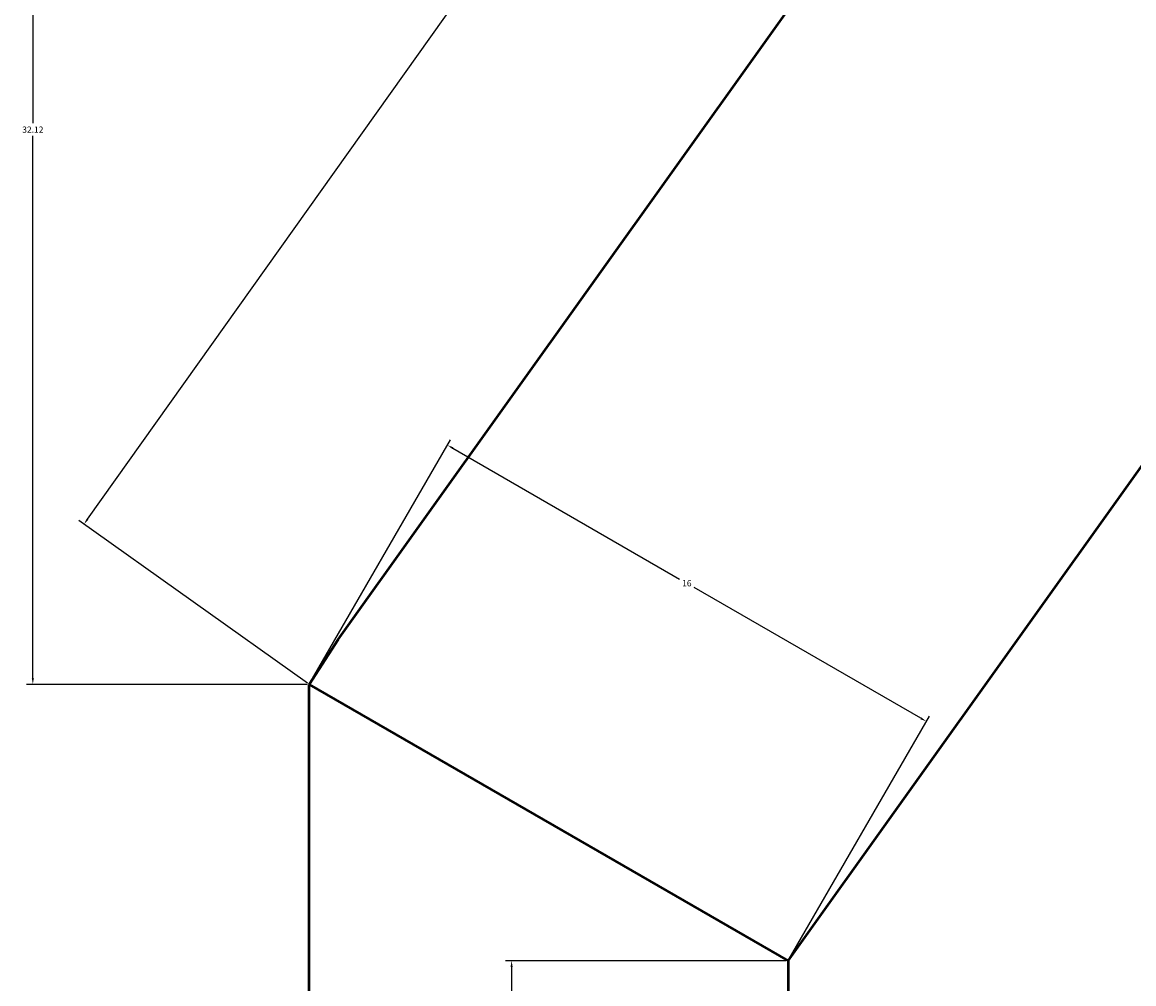
# Model space of a CAD drawing. Units: millimetres. Extents: x 2919 to 3075, y 2801 to 2951.
# Tile 3 of 14: x 2919 to 2952, y 2882 to 2910. Entities that reach past the tile are written whole.
import ezdxf

# ---------------------------------------------------------------- set-up
doc = ezdxf.new("R2010")
doc.units = ezdxf.units.MM
doc.layers.add('M-DIMS', color=2, linetype='Continuous', lineweight=18)
doc.layers.add('M-OUTL', color=7, linetype='Continuous', lineweight=50)
doc.styles.get("Standard").update_dxf_attribs({"font": 'arial.ttf'})
doc.dimstyles.get("Standard").update_dxf_attribs({"dimtxt": 0.18, "dimasz": 0.18, "dimexe": 0.18, "dimexo": 0.0625, "dimgap": 0.09, "dimtad": 0, "dimtih": 1, "dimtoh": 1, "dimdec": 4, "dimzin": 0, "dimdsep": 46, "dimtxsty": 'Standard', "dimcen": 0.09, "dimadec": 0, "dimazin": 0, "dimtfac": 1, "dimtdec": 4, "dimtofl": 0, "dimtmove": 0, "dimatfit": 3, "dimfxl": 1, "dimtolj": 1, "dimtzin": 0, "dimarcsym": 0})

# ---------------------------------------------------------------- blocks, each defined once
blk = doc.blocks.new('*D10')
at = {"layer": 'Defpoints', "color": 0, "transparency": 16777216}
for p in [(2956.682, 2882.821), (2960.682, 2875.893), (2941.63, 2864.893)]:
    blk.add_point(p, dxfattribs=at)
at = {"layer": 'M-DIMS', "color": 0, "lineweight": -2, "transparency": 16777216}
for p, q in [((2960.651, 2875.947), (2956.592, 2882.977)), ((2956.526, 2882.731), (2947.375, 2877.448)), ((2937.785, 2871.911), (2946.936, 2877.195)), ((2941.598, 2864.947), (2937.54, 2871.977))]:
    blk.add_line(p, q, dxfattribs=at)
at = {"layer": 'M-DIMS', "color": 0, "transparency": 16777216}
for points in [[(2956.511, 2882.757), (2956.541, 2882.705), (2956.682, 2882.821)], [(2937.77, 2871.937), (2937.8, 2871.885), (2937.63, 2871.821)]]:
    blk.add_solid(points, dxfattribs=at)
at = {"layer": 'M-DIMS', "color": 0, "transparency": 16777216, "insert": (2947.156, 2877.321), "char_height": 0.18, "attachment_point": 5}
blk.add_mtext('\\A1;22', dxfattribs=at)
blk = doc.blocks.new('*D14')
at = {"layer": 'Defpoints', "color": 0, "transparency": 16777216}
for p in [(2927.773, 2890.893), (2945.63, 2889.821), (2941.63, 2882.893)]:
    blk.add_point(p, dxfattribs=at)
at = {"layer": 'M-DIMS', "color": 0, "lineweight": -2, "transparency": 16777216}
for p, q in [((2927.804, 2890.947), (2931.863, 2897.977)), ((2931.929, 2897.731), (2938.491, 2893.943)), ((2945.474, 2889.911), (2938.912, 2893.7)), ((2941.661, 2882.947), (2945.72, 2889.977))]:
    blk.add_line(p, q, dxfattribs=at)
at = {"layer": 'M-DIMS', "color": 0, "transparency": 16777216}
for points in [[(2931.944, 2897.757), (2931.914, 2897.705), (2931.773, 2897.821)], [(2945.489, 2889.937), (2945.459, 2889.885), (2945.63, 2889.821)]]:
    blk.add_solid(points, dxfattribs=at)
at = {"layer": 'M-DIMS', "color": 0, "transparency": 16777216, "insert": (2938.701, 2893.821), "char_height": 0.18, "attachment_point": 5}
blk.add_mtext('\\A1;16', dxfattribs=at)
blk = doc.blocks.new('*D15')
at = {"layer": 'Defpoints', "color": 0, "transparency": 16777216}
for p in [(2933.63, 2882.893), (2941.63, 2882.893), (2941.63, 2864.893)]:
    blk.add_point(p, dxfattribs=at)
at = {"layer": 'M-DIMS', "color": 0, "lineweight": -2, "transparency": 16777216}
for p, q in [((2941.567, 2882.893), (2933.45, 2882.893)), ((2933.63, 2882.713), (2933.63, 2874.075)), ((2933.63, 2865.073), (2933.63, 2873.711)), ((2941.567, 2864.893), (2933.45, 2864.893))]:
    blk.add_line(p, q, dxfattribs=at)
at = {"layer": 'M-DIMS', "color": 0, "transparency": 16777216}
for points in [[(2933.6, 2882.713), (2933.66, 2882.713), (2933.63, 2882.893)], [(2933.6, 2865.073), (2933.66, 2865.073), (2933.63, 2864.893)]]:
    blk.add_solid(points, dxfattribs=at)
at = {"layer": 'M-DIMS', "color": 0, "transparency": 16777216, "insert": (2933.63, 2873.893), "char_height": 0.18, "attachment_point": 5}
blk.add_mtext('\\A1;18', dxfattribs=at)
blk = doc.blocks.new('*D21')
at = {"layer": 'Defpoints', "color": 0, "transparency": 16777216}
for p in [(2944.107, 2927.653), (2950.626, 2923.015), (2927.773, 2890.893)]:
    blk.add_point(p, dxfattribs=at)
at = {"layer": 'M-DIMS', "color": 0, "lineweight": -2, "transparency": 16777216}
for p, q in [((2950.575, 2923.052), (2943.961, 2927.757)), ((2944.003, 2927.506), (2932.81, 2911.774)), ((2921.359, 2895.677), (2932.551, 2911.41)), ((2927.722, 2890.929), (2921.108, 2895.635))]:
    blk.add_line(p, q, dxfattribs=at)
at = {"layer": 'M-DIMS', "color": 0, "transparency": 16777216}
for points in [[(2943.978, 2927.524), (2944.027, 2927.489), (2944.107, 2927.653)], [(2921.334, 2895.695), (2921.383, 2895.66), (2921.255, 2895.531)]]:
    blk.add_solid(points, dxfattribs=at)
at = {"layer": 'M-DIMS', "color": 0, "transparency": 16777216, "insert": (2932.681, 2911.592), "char_height": 0.18, "attachment_point": 5}
blk.add_mtext('\\A1;39.42', dxfattribs=at)
blk = doc.blocks.new('*D23')
at = {"layer": 'Defpoints', "color": 0, "transparency": 16777216}
for p in [(2919.773, 2923.015), (2950.626, 2923.015), (2927.773, 2890.893)]:
    blk.add_point(p, dxfattribs=at)
at = {"layer": 'M-DIMS', "color": 0, "lineweight": -2, "transparency": 16777216}
for p, q in [((2950.563, 2923.015), (2919.593, 2923.015)), ((2919.773, 2922.835), (2919.773, 2907.136)), ((2919.773, 2891.073), (2919.773, 2906.772)), ((2927.711, 2890.893), (2919.593, 2890.893))]:
    blk.add_line(p, q, dxfattribs=at)
at = {"layer": 'M-DIMS', "color": 0, "transparency": 16777216}
for points in [[(2919.743, 2922.835), (2919.803, 2922.835), (2919.773, 2923.015)], [(2919.743, 2891.073), (2919.803, 2891.073), (2919.773, 2890.893)]]:
    blk.add_solid(points, dxfattribs=at)
at = {"layer": 'M-DIMS', "color": 0, "transparency": 16777216, "insert": (2919.773, 2906.954), "char_height": 0.18, "attachment_point": 5}
blk.add_mtext('\\A1;32.12', dxfattribs=at)

msp = doc.modelspace()

# ---------------------------------------------------------------- linework, layer by layer
at = {"layer": 'M-OUTL'}
for p, q in [((2928.6099, 2892.1931), (2927.7732, 2890.8932)), ((2927.7732, 2856.8932), (2927.7732, 2890.8932)), ((2927.7732, 2890.8932), (2941.6296, 2882.8932)), ((2941.6296, 2882.8932), (2941.6296, 2864.8932))]:
    msp.add_line(p, q, dxfattribs=at)
for points in [[(2928.6099, 2892.1931), (2950.6258, 2923.0154), (2987.3232, 2944.2026)], [(2941.6296, 2882.8932), (2961.6296, 2910.8932), (2995.3232, 2930.3462)], [(2941.6296, 2882.8932), (2961.6296, 2910.8932), (2995.3232, 2930.3462)]]:
    msp.add_lwpolyline(points, dxfattribs=at)

# ---------------------------------------------------------------- dimensions: what is measured, and where the dimension line sits
at = {"layer": 'M-DIMS'}
for base, p1, p2, angle, override, picture, middle in [((2944.1072, 2927.653), (2927.7732, 2890.8932), (2950.6258, 2923.0154), 54.57085, {"dimdec": 2, "dimlfac": 1, "dimrnd": 0, "dimzin": 0, "dimdsep": 46, "dimlunit": 2}, '*D21', (2932.6808, 2911.5919)), ((2919.7732, 2923.0154), (2927.7732, 2890.8932), (2950.6258, 2923.0154), 90, {"dimdec": 2, "dimlfac": 1, "dimrnd": 0, "dimzin": 0, "dimdsep": 46, "dimlunit": 2}, '*D23', (2919.7732, 2906.9543)), ((2945.6296, 2889.8214), (2927.7732, 2890.8932), (2941.6296, 2882.8932), 330, {"dimdec": 0, "dimlfac": 1, "dimrnd": 0, "dimzin": 0, "dimdsep": 46, "dimlunit": 2}, '*D14', (2938.7014, 2893.8214)), ((2956.6821, 2882.8214), (2941.6296, 2864.8932), (2960.6821, 2875.8932), 30, {"dimdec": 0, "dimlfac": 1, "dimrnd": 0, "dimzin": 0, "dimdsep": 46, "dimlunit": 2}, '*D10', (2947.1559, 2877.3214)), ((2933.6296, 2882.8932), (2941.6296, 2864.8932), (2941.6296, 2882.8932), 90, {"dimdec": 0, "dimlfac": 1, "dimrnd": 0, "dimzin": 0, "dimdsep": 46, "dimlunit": 2}, '*D15', (2933.6296, 2873.8932))]:
    dim = msp.add_linear_dim(base=base, p1=p1, p2=p2, angle=angle, dimstyle='Standard', override=override, dxfattribs=at)
    dim.commit()
    dim.dimension.update_dxf_attribs({"geometry": picture, "text_midpoint": middle})

doc.saveas('drawing.dxf')
